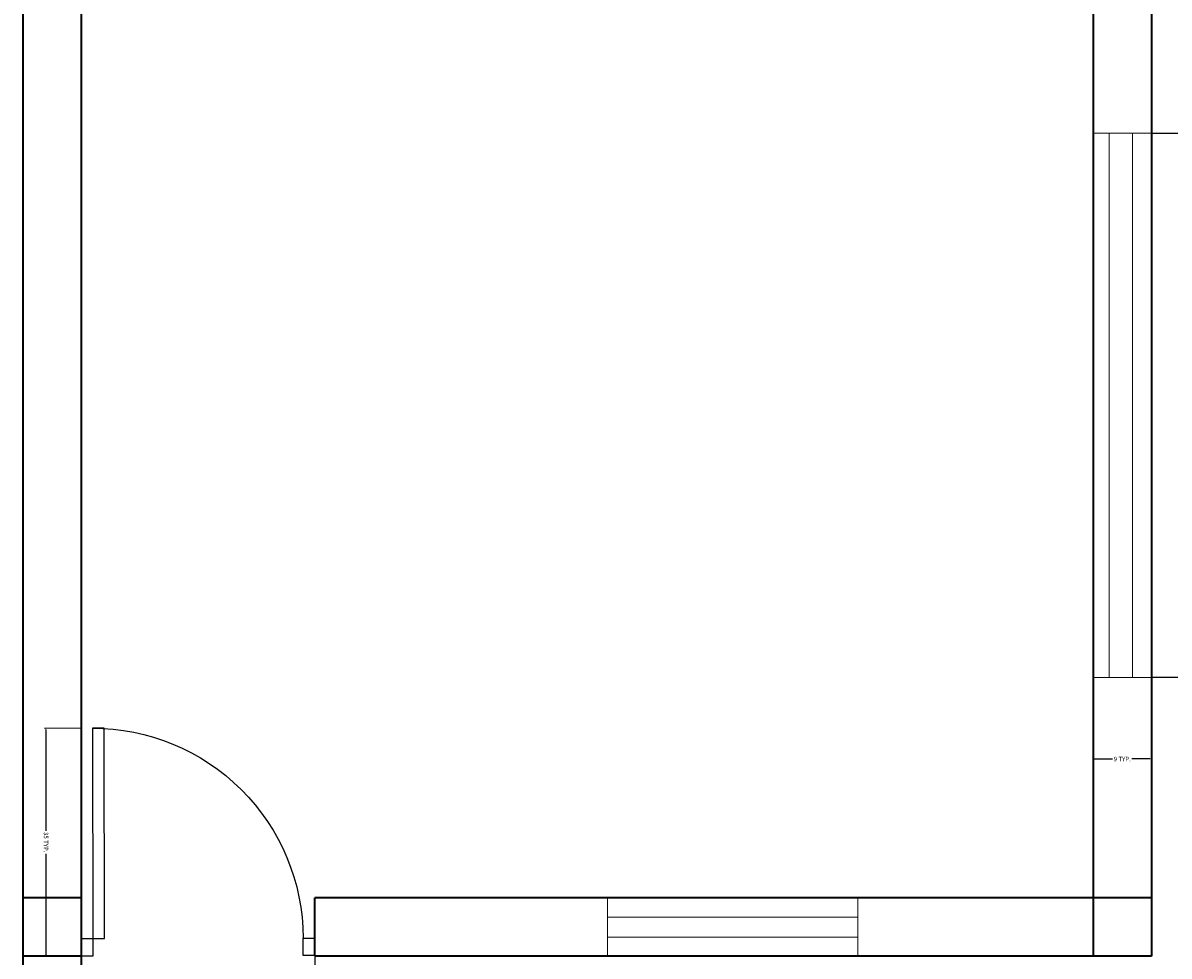
# Model space of a CAD drawing. Units: inches. Extents: x 867 to 1667, y -234 to 788.
# Tile 36 of 42: x 1395 to 1572, y 258 to 401. Entities that reach past the tile are written whole.
import ezdxf

# ---------------------------------------------------------------- set-up
doc = ezdxf.new("R2010")
doc.units = ezdxf.units.IN
doc.header["$MEASUREMENT"] = 0
for name, color, linetype, lineweight in [('A-ANNO-DIMS', 2, 'Continuous', 18), ('A-Door', 150, 'Continuous', 25), ('A-Glaz', 92, 'Continuous', 18), ('A-Wall', 7, 'Continuous', 35)]:
    doc.layers.add(name, color=color, linetype=linetype, lineweight=lineweight)
doc.layers.add('NET 01', color=8, linetype='Continuous')
doc.styles.get("Standard").update_dxf_attribs({"font": 'arial.ttf'})
doc.dimstyles.get("Standard").update_dxf_attribs({"dimtxt": 0.6875, "dimasz": 0.18, "dimexe": 0.18, "dimexo": 0.0625, "dimgap": 0.09, "dimtad": 0, "dimdec": 4, "dimzin": 0, "dimdsep": 46, "dimlunit": 4, "dimtxsty": 'Standard', "dimcen": 0.09, "dimadec": 0, "dimazin": 0, "dimtfac": 1, "dimtdec": 4, "dimtofl": 0, "dimtmove": 0, "dimatfit": 3, "dimfxl": 1, "dimtolj": 1, "dimtzin": 0, "dimarcsym": 0})

# ---------------------------------------------------------------- blocks, each defined once
blk = doc.blocks.new('A$C292B336C')
at = {"layer": 'A-Door'}
for points in [[(-0.05, 0), (-0.05, 0.9), (0, 0.9), (0, 0)], [(-0.95, 0), (-0.95, -0.075), (-0.9, -0.075), (-0.9, 0)], [(0, 0), (0, -0.075), (0.05, -0.075), (0.05, 0)]]:
    blk.add_lwpolyline(points, close=True, dxfattribs=at)
at = {"layer": 'NET 01'}
blk.add_arc((0, 0), 0.9, 90, 180, dxfattribs=at)
blk = doc.blocks.new('WIN-38_58IN')
for p, q in [((0, 9), (0, 0)), ((38.58, 0), (38.58, 9)), ((0, 6), (38.58, 6)), ((0, 2.92), (38.58, 2.92)), ((0, 0), (38.58, 0))]:
    blk.add_line(p, q)
blk = doc.blocks.new('WIN-83_90IN')
for p, q in [((0, 83.9), (9, 83.9)), ((2.51, 83.9), (2.51, 0)), ((6.08, 0), (6.08, 83.9)), ((0, 0), (9, 0))]:
    blk.add_line(p, q)
blk = doc.blocks.new('*D5')
at = {"layer": 'A-ANNO-DIMS', "color": 0, "lineweight": -2, "transparency": 16777216}
for p, q in [((1403.89, 257.55), (1403.9, 252.04)), ((1439.9, 257.64), (1439.91, 252.12)), ((1404.08, 252.22), (1418.58, 252.25)), ((1439.73, 252.3), (1425.22, 252.26))]:
    blk.add_line(p, q, dxfattribs=at)
at = {"layer": 'A-ANNO-DIMS', "color": 0, "transparency": 16777216}
for points in [[(1404.08, 252.25), (1404.08, 252.19), (1403.9, 252.22)], [(1439.73, 252.33), (1439.73, 252.27), (1439.91, 252.3)]]:
    blk.add_solid(points, dxfattribs=at)
at = {"layer": 'Defpoints', "color": 0, "transparency": 16777216}
for p in [(1403.89, 257.62), (1439.9, 257.7), (1403.9, 252.22)]:
    blk.add_point(p, dxfattribs=at)
at = {"layer": 'A-ANNO-DIMS', "color": 0, "transparency": 16777216, "insert": (1421.9, 252.26), "char_height": 0.6875, "attachment_point": 5, "rotation": 0.1281}
blk.add_mtext('\\A1;DOOR 36 TYP.', dxfattribs=at)
blk = doc.blocks.new('*D6')
at = {"layer": 'A-ANNO-DIMS', "color": 0, "lineweight": -2, "transparency": 16777216}
for p, q in [((1403.75, 292.73), (1398.23, 292.72)), ((1398.41, 292.54), (1398.44, 276.92)), ((1398.48, 257.78), (1398.45, 273.4)), ((1403.82, 257.62), (1398.3, 257.6))]:
    blk.add_line(p, q, dxfattribs=at)
at = {"layer": 'A-ANNO-DIMS', "color": 0, "transparency": 16777216}
for points in [[(1398.44, 292.54), (1398.38, 292.54), (1398.41, 292.72)], [(1398.51, 257.78), (1398.45, 257.78), (1398.48, 257.6)]]:
    blk.add_solid(points, dxfattribs=at)
at = {"layer": 'Defpoints', "color": 0, "transparency": 16777216}
for p in [(1398.41, 292.72), (1403.81, 292.73), (1403.89, 257.62)]:
    blk.add_point(p, dxfattribs=at)
at = {"layer": 'A-ANNO-DIMS', "color": 0, "transparency": 16777216, "insert": (1398.45, 275.16), "char_height": 0.6875, "attachment_point": 5, "rotation": 270.1281}
blk.add_mtext('\\A1;35 TYP.', dxfattribs=at)
blk = doc.blocks.new('*D15')
at = {"layer": 'A-ANNO-DIMS', "color": 0, "lineweight": -2, "transparency": 16777216}
for p, q in [((1568.95, 384.49), (1581.65, 384.49)), ((1581.47, 384.31), (1581.47, 346.55)), ((1581.47, 300.77), (1581.47, 338.52)), ((1568.95, 300.59), (1581.65, 300.59))]:
    blk.add_line(p, q, dxfattribs=at)
at = {"layer": 'A-ANNO-DIMS', "color": 0, "transparency": 16777216}
for points in [[(1581.44, 384.31), (1581.5, 384.31), (1581.47, 384.49)], [(1581.44, 300.77), (1581.5, 300.77), (1581.47, 300.59)]]:
    blk.add_solid(points, dxfattribs=at)
at = {"layer": 'Defpoints', "color": 0, "transparency": 16777216}
for p in [(1568.89, 384.49), (1581.47, 384.49), (1568.89, 300.59)]:
    blk.add_point(p, dxfattribs=at)
at = {"layer": 'A-ANNO-DIMS', "color": 0, "transparency": 16777216, "insert": (1581.47, 342.54), "char_height": 0.6875, "attachment_point": 5, "rotation": 90}
blk.add_mtext('\\A1;WINDOW 84 TYP.', dxfattribs=at)
blk = doc.blocks.new('*D16')
at = {"layer": 'A-ANNO-DIMS', "color": 0, "lineweight": -2, "transparency": 16777216}
for p, q in [((1559.89, 300.52), (1559.89, 287.82)), ((1568.89, 300.52), (1568.89, 287.82)), ((1560.07, 288), (1562.89, 288)), ((1568.71, 288), (1565.88, 288))]:
    blk.add_line(p, q, dxfattribs=at)
at = {"layer": 'A-ANNO-DIMS', "color": 0, "transparency": 16777216}
for points in [[(1560.07, 288.03), (1560.07, 287.97), (1559.89, 288)], [(1568.71, 288.03), (1568.71, 287.97), (1568.89, 288)]]:
    blk.add_solid(points, dxfattribs=at)
at = {"layer": 'Defpoints', "color": 0, "transparency": 16777216}
for p in [(1559.89, 300.59), (1568.89, 300.59), (1568.89, 288)]:
    blk.add_point(p, dxfattribs=at)
at = {"layer": 'A-ANNO-DIMS', "color": 0, "transparency": 16777216, "insert": (1564.39, 288), "char_height": 0.688, "attachment_point": 5}
blk.add_mtext('\\A1;9 TYP.', dxfattribs=at)

msp = doc.modelspace()

# ---------------------------------------------------------------- linework, layer by layer
at = {"layer": 'A-Wall'}
for p, q in [((1394.8866, 413.617), (1394.8866, 136.117)), ((1403.8866, 413.617), (1403.8866, 136.117)), ((1568.8866, 413.617), (1568.8866, 257.617)), ((1559.8866, 404.617), (1559.8866, 257.617)), ((1403.8866, 266.617), (1394.8866, 266.617)), ((1568.8866, 266.617), (1439.8783, 266.617)), ((1439.8983, 257.6976), (1439.8783, 266.617)), ((1403.8866, 257.617), (1394.8866, 257.617)), ((1568.8866, 257.617), (1439.8783, 257.617))]:
    msp.add_line(p, q, dxfattribs=at)

# ---------------------------------------------------------------- block references
at = {"layer": 'A-Door', "xscale": -36.01171521992244, "yscale": 36.01171521992244, "zscale": 36.01171521992244, "rotation": 0.1281311246168038}
msp.add_blockref('A$C292B336C', (1405.6812, 260.3219), dxfattribs=at)
at = {"layer": 'A-Glaz'}
for name, p in [('WIN-83_90IN', (1559.887, 300.5855)), ('WIN-38_58IN', (1485.0208, 257.617))]:
    msp.add_blockref(name, p, dxfattribs=at)

# ---------------------------------------------------------------- dimensions: what is measured, and where the dimension line sits
at = {"layer": 'A-ANNO-DIMS'}
for base, p1, p2, angle, text, picture, middle in [((1581.472, 384.4878), (1568.8866, 300.5856), (1568.8866, 384.4878), 90, 'WINDOW <> TYP.', '*D15', (1581.472, 342.5367)), ((1398.4064, 292.7163), (1403.8866, 257.617), (1403.8081, 292.7284), 90.128131, '<> TYP.', '*D6', (1398.4456, 275.1606)), ((1403.8987, 252.2153), (1439.8983, 257.6976), (1403.8866, 257.617), 180.128131, 'DOOR <> TYP.', '*D5', (1421.9045, 252.2556))]:
    dim = msp.add_linear_dim(base=base, p1=p1, p2=p2, angle=angle, text=text, dimstyle='Standard', override={"dimdec": 0, "dimlfac": 1, "dimrnd": 0, "dimzin": 0, "dimdsep": 46, "dimlunit": 2}, dxfattribs=at)
    dim.commit()
    dim.dimension.update_dxf_attribs({"geometry": picture, "text_midpoint": middle})
dim = msp.add_linear_dim(base=(1568.8866, 288.0003), p1=(1559.8866, 300.5856), p2=(1568.8866, 300.5856), text='<> TYP.', dimstyle='Standard', override={"dimdec": 0, "dimlfac": 1, "dimrnd": 0, "dimzin": 0, "dimdsep": 46, "dimlunit": 2}, dxfattribs=at)
dim.commit()
dim.dimension.update_dxf_attribs({"geometry": '*D16', "text_midpoint": (1564.3866, 288.0003)})

doc.saveas('drawing.dxf')
